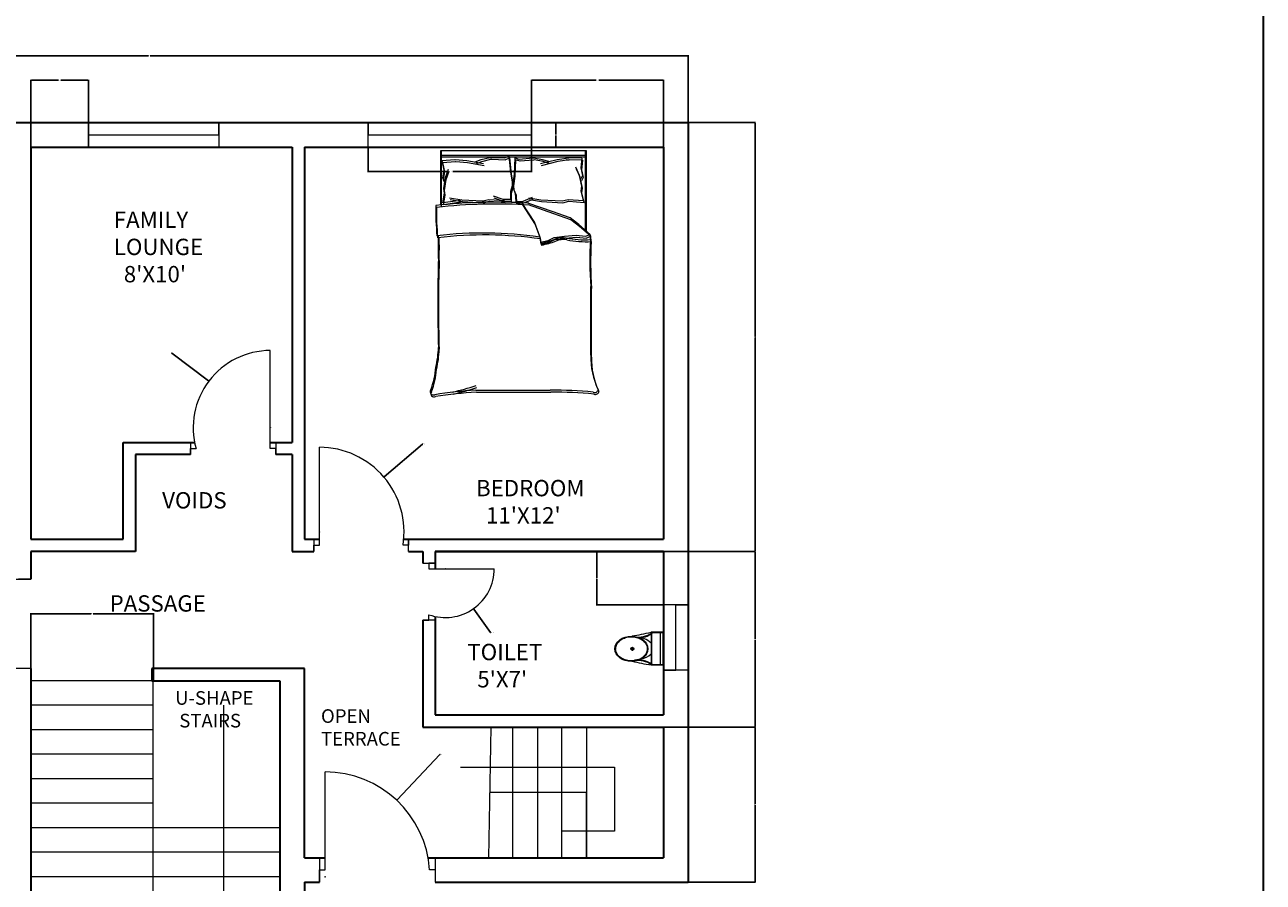
# Model space of a CAD drawing. Units: inches. Extents: x 2067 to 3463, y 1605 to 2723.
# Tile 10 of 10: x 3008 to 3463, y 1879 to 2194. Entities that reach past the tile are written whole.
import ezdxf

# ---------------------------------------------------------------- set-up
doc = ezdxf.new("R2010")
doc.units = ezdxf.units.IN
for name, color, linetype, lineweight in [('A-ANNO-DIMS', 2, 'Continuous', 18), ('A-ANNO-TTLB', 7, 'Continuous', 35), ('A-AREA-IDEN', 7, 'Continuous', 18), ('A-DOOR', 3, 'Continuous', 18), ('A-FLOR-FIXT', 8, 'Continuous', 18), ('A-FLOR-STRS', 7, 'Continuous', 18), ('A-FURN', 8, 'Continuous', 13), ('A-GLAZ', 4, 'Continuous', 18), ('A-WALL', 7, 'Continuous', 35)]:
    doc.layers.add(name, color=color, linetype=linetype, lineweight=lineweight)
doc.styles.get("Standard").update_dxf_attribs({"font": 'arial.ttf'})
doc.dimstyles.get("Standard").update_dxf_attribs({"dimtxt": 0.18, "dimasz": 0.18, "dimexe": 0.18, "dimexo": 0.0625, "dimgap": 0.09, "dimtad": 0, "dimtih": 1, "dimtoh": 1, "dimdec": 4, "dimzin": 0, "dimdsep": 46, "dimtxsty": 'Standard', "dimcen": 0.09, "dimadec": 0, "dimazin": 0, "dimtfac": 1, "dimtdec": 4, "dimtofl": 0, "dimtmove": 0, "dimatfit": 3, "dimfxl": 1, "dimtolj": 1, "dimtzin": 0, "dimarcsym": 0})

# ---------------------------------------------------------------- blocks, each defined once
blk = doc.blocks.new('A$C31115884')
for p, q in [((283, 498), (223, 498)), ((258, 466), (258, 523)), ((0, 200), (0, 0)), ((520, 200), (0, 200)), ((520, 0), (520, 200)), ((510, 54), (0, 54)), ((10, 190), (10, 10)), ((510, 190), (10, 190)), ((10, 10), (510, 10)), ((510, 10), (510, 190)), ((0, 0), (520, 0))]:
    blk.add_line(p, q)
blk.add_circle((256, 496), 23.6)
for centre, radius, start, end in [((2778, -205), 2807, 165.4549, 171.7133), ((-295, 403), 365, 324.2091, 9.3499), ((-295, 403), 375, 324.2091, 9.3499), ((139, 406), 293, 315.8436, 2.6563), ((806, 403), 375, 179.2036, 215.7909), ((806, 403), 365, 170.6501, 215.7909), ((3237, 905), 2807, 188.2867, 194.5451), ((384, 406), 293, 190.2774, 224.1564)]:
    blk.add_arc(centre, radius, start, end)
blk.add_ellipse((256, 510), major_axis=(0, -261), ratio=0.772727)
blk.add_open_spline([(256, 259), (263, 259), (270, 260), (288, 262), (299, 265), (320, 273), (330, 278), (350, 291), (360, 299), (378, 316), (386, 326), (402, 347), (409, 358), (421, 383), (427, 395), (436, 422), (440, 436), (445, 465), (447, 480), (448, 509), (448, 524), (445, 553), (443, 568), (436, 596), (432, 610), (422, 636), (416, 649), (402, 672), (395, 683), (379, 703), (370, 712), (351, 728), (341, 735), (321, 746), (310, 751), (289, 757), (278, 759), (256, 761), (245, 761), (223, 757), (212, 754), (191, 746), (181, 741), (161, 728), (151, 720), (133, 703), (125, 693), (110, 672), (103, 660), (90, 636), (85, 623), (76, 596), (72, 582), (67, 553), (66, 538), (64, 509), (65, 494), (68, 465), (70, 450), (77, 422), (81, 408), (91, 382), (97, 370), (111, 346), (118, 335), (135, 316), (144, 307), (162, 291), (172, 284), (193, 273), (203, 269), (225, 262), (236, 260), (250, 259), (253, 259), (256, 259)], degree=3, knots=[0, 0, 0, 0, 0.110105, 0.110105, 0.285049, 0.285049, 0.459994, 0.459994, 0.634938, 0.634938, 0.809882, 0.809882, 0.984827, 0.984827, 1.159771, 1.159771, 1.334715, 1.334715, 1.50966, 1.50966, 1.684604, 1.684604, 1.859549, 1.859549, 2.034493, 2.034493, 2.209437, 2.209437, 2.384382, 2.384382, 2.559326, 2.559326, 2.73427, 2.73427, 2.909215, 2.909215, 3.084159, 3.084159, 3.259103, 3.259103, 3.434048, 3.434048, 3.608992, 3.608992, 3.783936, 3.783936, 3.958881, 3.958881, 4.133825, 4.133825, 4.30877, 4.30877, 4.483714, 4.483714, 4.658658, 4.658658, 4.833603, 4.833603, 5.008547, 5.008547, 5.183491, 5.183491, 5.358436, 5.358436, 5.53338, 5.53338, 5.708324, 5.708324, 5.883269, 5.883269, 6.058213, 6.058213, 6.233158, 6.233158, 6.283185, 6.283185, 6.283185, 6.283185])
blk = doc.blocks.new('BED-DOUBLE')
for p, q in [((3.86, 70.43), (3.86, 90.57)), ((3.86, 90.57), (57.01, 90.57)), ((3.86, 88.86), (57.01, 88.86)), ((4.12, 89.85), (4.12, 90.57)), ((4.12, 69.72), (4.12, 89.85)), ((4.12, 88.15), (57.26, 88.15)), ((4.33, 86.88), (4.97, 83.34)), ((4.34, 86.85), (9.1, 87.22)), ((4.59, 86.14), (9.35, 86.51)), ((9.1, 87.22), (9.21, 87.2)), ((9.21, 87.2), (13.46, 86.88)), ((9.35, 86.51), (9.47, 86.49)), ((9.47, 86.49), (13.72, 86.17)), ((13.46, 86.88), (19.57, 85.75)), ((16.52, 86.4), (18.77, 87.2)), ((16.77, 85.68), (19.02, 86.49)), ((18.77, 87.2), (21.98, 88)), ((19.02, 86.49), (22.24, 87.29)), ((21.98, 88), (22.34, 88)), ((22.24, 87.29), (22.6, 87.29)), ((22.34, 88), (27.29, 87.84)), ((22.6, 87.29), (27.54, 87.13)), ((27.29, 87.84), (28.89, 88.49)), ((27.54, 87.13), (29.15, 87.77)), ((28.89, 88.49), (29.54, 82.54)), ((29.15, 87.77), (29.79, 81.83)), ((31.11, 87.79), (30.84, 81.82)), ((31.36, 87.08), (31.09, 81.11)), ((32.76, 87.25), (31.11, 87.79)), ((33.01, 86.54), (31.36, 87.08)), ((37.68, 87.72), (32.76, 87.25)), ((37.93, 87.01), (33.01, 86.54)), ((38.04, 87.74), (37.68, 87.72)), ((38.29, 87.03), (37.93, 87.01)), ((41.29, 87.14), (38.04, 87.74)), ((41.55, 86.43), (38.29, 87.03)), ((46.61, 87.15), (40.58, 85.65)), ((43.59, 86.48), (41.29, 87.14)), ((50.83, 87.74), (46.61, 87.15)), ((51.09, 87.03), (46.86, 86.44)), ((55.73, 87.72), (49.72, 87.83)), ((49.72, 87.83), (50.83, 87.74)), ((55.98, 87.01), (49.97, 87.12)), ((49.97, 87.12), (51.09, 87.03)), ((55.73, 87.72), (55.3, 84.15)), ((55.98, 87.01), (55.56, 83.44)), ((57.01, 90.57), (57.01, 60.97)), ((57.01, 90.57), (57.26, 90.57)), ((57.26, 90.57), (57.26, 89.74)), ((57.26, 89.85), (57.26, 60.26)), ((4.97, 83.34), (4.49, 80.45)), ((4.59, 86.17), (5.23, 82.63)), ((5.23, 82.63), (4.75, 79.74)), ((5.62, 80.61), (6.74, 83.66)), ((5.87, 79.9), (7, 82.95)), ((13.72, 86.17), (19.83, 85.04)), ((29.54, 82.54), (30.18, 79)), ((46.86, 86.44), (40.84, 84.94)), ((43.85, 85.77), (41.55, 86.43)), ((54.83, 81.38), (53.52, 84.36)), ((55.09, 80.67), (53.77, 83.65)), ((55.3, 84.15), (55.97, 81.29)), ((55.56, 83.44), (56.22, 80.58)), ((4.49, 80.45), (5.13, 79.32)), ((4.75, 79.74), (5.39, 78.61)), ((4.97, 76.59), (5.62, 80.61)), ((5.23, 75.88), (5.87, 79.9)), ((30.18, 77.55), (29.54, 75.46)), ((29.79, 81.83), (30.43, 78.29)), ((30.18, 79), (30.18, 77.55)), ((30.84, 81.82), (30.42, 78.25)), ((30.42, 78.25), (30.51, 76.8)), ((30.43, 78.29), (30.43, 76.84)), ((31.09, 81.11), (30.67, 77.54)), ((30.67, 77.54), (30.76, 76.09)), ((55.73, 77.41), (54.83, 81.38)), ((55.98, 76.7), (55.09, 80.67)), ((55.97, 81.29), (55.39, 80.13)), ((55.51, 75.63), (55.73, 77.41)), ((56.22, 80.58), (55.65, 79.42)), ((4.65, 71.28), (5.3, 74.82)), ((4.91, 70.57), (5.55, 74.11)), ((5.3, 74.82), (4.97, 76.59)), ((5.55, 74.11), (5.23, 75.88)), ((7.1, 73.19), (11.58, 72.44)), ((26.8, 72.48), (23.31, 73.69)), ((27.06, 71.77), (23.56, 72.98)), ((29.54, 75.46), (29.54, 72.48)), ((30.43, 76.84), (29.79, 74.75)), ((29.79, 74.75), (29.79, 71.77)), ((30.51, 76.8), (31.28, 74.76)), ((30.76, 76.09), (31.54, 74.05)), ((31.28, 74.76), (31.47, 71.78)), ((31.54, 74.05), (31.72, 71.07)), ((34.19, 71.95), (37.61, 73.38)), ((36.21, 73.19), (40.7, 72.44)), ((56.38, 72.14), (55.51, 75.63)), ((55.77, 74.92), (55.98, 76.7)), ((56.63, 71.43), (55.77, 74.92)), ((10.32, 72.09), (4.65, 71.28)), ((10.57, 71.37), (4.91, 70.57)), ((7.35, 72.48), (11.83, 71.73)), ((11.58, 72.44), (10.32, 72.09)), ((11.83, 71.73), (10.57, 71.37)), ((11.58, 72.44), (19.38, 71.97)), ((11.83, 71.73), (19.63, 71.25)), ((19.38, 71.97), (21.56, 72.58)), ((19.63, 71.25), (21.81, 71.87)), ((21.56, 72.58), (27.26, 72.14)), ((21.81, 71.87), (27.52, 71.43)), ((29.54, 72.48), (26.8, 72.48)), ((29.79, 71.77), (27.06, 71.77)), ((31.47, 71.78), (34.19, 71.95)), ((31.72, 71.07), (34.45, 71.24)), ((33.65, 71.23), (38.31, 64.01)), ((33.9, 70.52), (38.56, 63.3)), ((34.45, 71.24), (37.86, 72.67)), ((45.2, 67.97), (35.92, 71.23)), ((45.45, 67.26), (36.18, 70.52)), ((36.47, 72.48), (40.95, 71.73)), ((40.7, 72.44), (48.49, 71.97)), ((40.95, 71.73), (48.74, 71.25)), ((48.49, 71.97), (50.67, 72.58)), ((48.74, 71.25), (50.92, 71.87)), ((50.67, 72.58), (56.38, 72.14)), ((50.92, 71.87), (56.63, 71.43)), ((38.31, 64.01), (40.2, 59.02)), ((51.4, 65.74), (45.2, 67.97)), ((51.65, 65.02), (45.45, 67.26)), ((54.67, 63.33), (51.4, 65.74)), ((54.92, 62.61), (51.65, 65.02)), ((38.56, 63.3), (40.46, 58.31)), ((49.33, 59.02), (53.64, 59.37)), ((53.64, 59.37), (57.08, 59.02)), ((58.79, 59.71), (54.67, 63.33)), ((59.04, 59), (54.92, 62.61)), ((57.08, 59.02), (58.79, 59.71)), ((58.88, 57.77), (58.79, 59.71, 4.3)), ((40.2, 59.02), (40.55, 56.79)), ((40.46, 58.31), (40.8, 56.07)), ((40.55, 56.79), (43.3, 57.47)), ((40.8, 56.07), (43.56, 56.76)), ((43.3, 57.47), (45.54, 58.51)), ((43.56, 56.76), (45.8, 57.8)), ((45.54, 58.51), (49.33, 59.02)), ((45.8, 57.8), (49.58, 58.31)), ((49.58, 58.31), (53.89, 58.66)), ((53.89, 58.66), (57.33, 58.31)), ((57.33, 58.31), (59.04, 59)), ((59.13, 57.06), (59.04, 59, 4.3)), ((16.75, 2.44), (44.12, 2.44)), ((17, 1.73), (44.38, 1.73))]:
    blk.add_line(p, q)
for centre, radius, start, end in [((94.7, 68.22), 92.64, 178.7218, 185.604), ((23.75, -111.88), 183.45, 86.0865, 96.7821), ((94.95, 67.51), 92.64, 178.7218, 185.604), ((24.01, -112.59), 183.45, 86.0865, 96.7821), ((19.74, -83.26), 143.47, 81.7845, 96.9006), ((20, -83.97), 143.47, 81.7845, 96.9006), ((-186.05, 55.9), 189.16, 358.4762, 1.0082), ((-185.79, 55.19), 189.16, 358.4762, 1.0082), ((40.74, 56.72), 0.205, 160.2464, 271.1377), ((34.64, 88.92), 32.98, 280.6617, 289.8806), ((40.99, 56.01), 0.205, 160.2464, 271.1377), ((34.9, 88.21), 32.98, 280.6617, 289.8806), ((48.64, 51.57), 6.92, 78.6608, 113.7384), ((48.9, 50.86), 6.92, 78.6608, 113.7384), ((57.08, 97.97), 40.24, 259.8763, 272.5657), ((57.33, 97.26), 40.24, 259.8763, 272.5657), ((202.68, 50.18), 144, 176.9791, 183.8365), ((202.94, 49.47), 144, 176.9791, 183.8365), ((539.13, 34.28), 536.33, 178.2277, 181.7185), ((539.38, 33.57), 536.33, 178.2277, 181.7185), ((-5013.77, 15.15), 5072.83, 0.00217, 0.28689), ((-5013.52, 14.44), 5072.83, 0.00217, 0.28689), ((-29.91, 18.82), 32.95, 346.0648, 358.9113), ((-29.66, 18.11), 32.95, 346.0648, 358.9113), ((84.69, 14.21), 25.65, 177.4714, 206.4681), ((84.94, 13.5), 25.65, 177.4714, 206.4681), ((-24.09, 12.42), 26.2, 337.9751, 356.652), ((-23.83, 11.71), 26.2, 337.9751, 356.652), ((1.21, 1.92), 1.21, 146.1736, 293.4781), ((1.46, 1.21), 1.21, 146.1736, 293.4781), ((23.83, -132.77), 135.4, 92.9958, 99.4091), ((24.08, -133.48), 135.4, 92.9958, 99.4091), ((-19.15, 116.93), 118.38, 283.3832, 287.7053), ((-18.9, 116.22), 118.38, 283.3832, 287.7053), ((45.76, -145.49), 147.94, 84.4998, 90.6351), ((46.02, -146.2), 147.94, 84.4998, 90.6351), ((60.5, 2.86), 1.23, 242.6588, 356.02), ((60.76, 2.15), 1.23, 242.6588, 356.02)]:
    blk.add_arc(centre, radius, start, end)
blk = doc.blocks.new('WIN-PLAN-24-OFFSET')
for p, q in [((0, 24), (9, 24)), ((9, 24), (4.5, 24)), ((4.5, 24), (4.5, 0)), ((4.5, 0), (0, 0)), ((0, 0), (9, 0))]:
    blk.add_line(p, q)
blk = doc.blocks.new('WIN-PLAN-48-OFFSET')
for p, q in [((0, 9), (0, 0)), ((48, 4.5), (48, 9)), ((48, 9), (48, 0)), ((0, 0), (0, 4.5)), ((0, 4.5), (48, 4.5))]:
    blk.add_line(p, q)
blk = doc.blocks.new('WIN-PLAN-60-ALIGNED')
for p, q in [((0, 0), (0, 9)), ((0, 9), (0, 4.5)), ((60, 4.5), (60, 9)), ((60, 9), (60, 0)), ((0, 4.5), (60, 4.5))]:
    blk.add_line(p, q)
blk = doc.blocks.new('*D24')
at = {"layer": 'A-ANNO-DIMS', "color": 0, "lineweight": -2, "transparency": 16777216}
for p, q in [((3134.41, 2149.17), (3134.41, 2140.05)), ((3194.41, 2149.17), (3194.41, 2140.05)), ((3134.59, 2140.23), (3163.3, 2140.23)), ((3194.23, 2140.23), (3165.53, 2140.23))]:
    blk.add_line(p, q, dxfattribs=at)
at = {"layer": 'A-ANNO-DIMS', "color": 0, "transparency": 16777216}
for points in [[(3134.59, 2140.26), (3134.59, 2140.2), (3134.41, 2140.23)], [(3194.23, 2140.26), (3194.23, 2140.2), (3194.41, 2140.23)]]:
    blk.add_solid(points, dxfattribs=at)
at = {"layer": 'Defpoints', "color": 0, "transparency": 16777216}
for p in [(3134.41, 2149.23), (3194.41, 2149.23), (3194.41, 2140.23)]:
    blk.add_point(p, dxfattribs=at)
at = {"layer": 'A-ANNO-DIMS', "color": 0, "transparency": 16777216, "insert": (3164.41, 2140.23), "char_height": 0.18, "attachment_point": 5}
blk.add_mtext('\\A1;WINDOW 60 TYP.', dxfattribs=at)
blk = doc.blocks.new('*D25')
at = {"layer": 'A-ANNO-DIMS', "color": 0, "lineweight": -2, "transparency": 16777216}
for p, q in [((3194.48, 2158.23), (3203.59, 2158.23)), ((3203.41, 2158.05), (3203.41, 2153.91)), ((3203.41, 2149.41), (3203.41, 2153.55)), ((3194.48, 2149.23), (3203.59, 2149.23))]:
    blk.add_line(p, q, dxfattribs=at)
at = {"layer": 'A-ANNO-DIMS', "color": 0, "transparency": 16777216}
for points in [[(3203.38, 2158.05), (3203.44, 2158.05), (3203.41, 2158.23)], [(3203.38, 2149.41), (3203.44, 2149.41), (3203.41, 2149.23)]]:
    blk.add_solid(points, dxfattribs=at)
at = {"layer": 'Defpoints', "color": 0, "transparency": 16777216}
for p in [(3194.41, 2158.23), (3203.41, 2158.23), (3194.41, 2149.23)]:
    blk.add_point(p, dxfattribs=at)
at = {"layer": 'A-ANNO-DIMS', "color": 0, "transparency": 16777216, "insert": (3203.41, 2153.73), "char_height": 0.18, "attachment_point": 5}
blk.add_mtext('\\A1;9 TYP.', dxfattribs=at)
blk = doc.blocks.new('*D50')
at = {"layer": 'A-ANNO-DIMS', "color": 0, "lineweight": -2, "transparency": 16777216}
for p, q in [((2856, 2158.29), (2856, 2183.01)), ((2856.18, 2182.83), (3053.71, 2182.83)), ((3251.82, 2182.83), (3054.29, 2182.83)), ((3252, 2158.29), (3252, 2183.01))]:
    blk.add_line(p, q, dxfattribs=at)
at = {"layer": 'A-ANNO-DIMS', "color": 0, "transparency": 16777216}
for points in [[(2856.18, 2182.86), (2856.18, 2182.8), (2856, 2182.83)], [(3251.82, 2182.86), (3251.82, 2182.8), (3252, 2182.83)]]:
    blk.add_solid(points, dxfattribs=at)
at = {"layer": 'Defpoints', "color": 0, "transparency": 16777216}
for p in [(3252, 2182.83), (2856, 2158.23), (3252, 2158.23)]:
    blk.add_point(p, dxfattribs=at)
at = {"layer": 'A-ANNO-DIMS', "color": 0, "transparency": 16777216, "insert": (3054, 2182.83), "char_height": 0.18, "attachment_point": 5}
blk.add_mtext('\\A1;396', dxfattribs=at)
blk = doc.blocks.new('*D58')
at = {"layer": 'A-ANNO-DIMS', "color": 0, "lineweight": -2, "transparency": 16777216}
for p, q in [((3252.06, 2158.23), (3276.78, 2158.23)), ((3276.6, 2158.05), (3276.6, 2079.66)), ((3276.6, 2000.91), (3276.6, 2079.3)), ((3243.06, 2000.73), (3276.78, 2000.73))]:
    blk.add_line(p, q, dxfattribs=at)
at = {"layer": 'A-ANNO-DIMS', "color": 0, "transparency": 16777216}
for points in [[(3276.57, 2158.05), (3276.63, 2158.05), (3276.6, 2158.23)], [(3276.57, 2000.91), (3276.63, 2000.91), (3276.6, 2000.73)]]:
    blk.add_solid(points, dxfattribs=at)
at = {"layer": 'Defpoints', "color": 0, "transparency": 16777216}
for p in [(3252, 2158.23), (3243, 2000.73), (3276.6, 2000.73)]:
    blk.add_point(p, dxfattribs=at)
at = {"layer": 'A-ANNO-DIMS', "color": 0, "transparency": 16777216, "insert": (3276.6, 2079.48), "char_height": 0.18, "attachment_point": 5}
blk.add_mtext('\\A1;157.5', dxfattribs=at)
blk = doc.blocks.new('*D59')
at = {"layer": 'A-ANNO-DIMS', "color": 0, "lineweight": -2, "transparency": 16777216}
for p, q in [((3243.06, 2000.73), (3276.78, 2000.73)), ((3276.6, 2000.55), (3276.6, 1968.66)), ((3276.6, 1936.41), (3276.6, 1968.3)), ((3243.06, 1936.23), (3276.78, 1936.23))]:
    blk.add_line(p, q, dxfattribs=at)
at = {"layer": 'A-ANNO-DIMS', "color": 0, "transparency": 16777216}
for points in [[(3276.57, 2000.55), (3276.63, 2000.55), (3276.6, 2000.73)], [(3276.57, 1936.41), (3276.63, 1936.41), (3276.6, 1936.23)]]:
    blk.add_solid(points, dxfattribs=at)
at = {"layer": 'Defpoints', "color": 0, "transparency": 16777216}
for p in [(3243, 2000.73), (3243, 1936.23), (3276.6, 1936.23)]:
    blk.add_point(p, dxfattribs=at)
at = {"layer": 'A-ANNO-DIMS', "color": 0, "transparency": 16777216, "insert": (3276.6, 1968.48), "char_height": 0.18, "attachment_point": 5}
blk.add_mtext('\\A1;64.5', dxfattribs=at)
blk = doc.blocks.new('*D60')
at = {"layer": 'A-ANNO-DIMS', "color": 0, "lineweight": -2, "transparency": 16777216}
for p, q in [((3243.06, 1936.23), (3276.78, 1936.23)), ((3276.6, 1936.05), (3276.6, 1907.91)), ((3276.6, 1879.41), (3276.6, 1907.55)), ((3252.06, 1879.23), (3276.78, 1879.23))]:
    blk.add_line(p, q, dxfattribs=at)
at = {"layer": 'A-ANNO-DIMS', "color": 0, "transparency": 16777216}
for points in [[(3276.57, 1936.05), (3276.63, 1936.05), (3276.6, 1936.23)], [(3276.57, 1879.41), (3276.63, 1879.41), (3276.6, 1879.23)]]:
    blk.add_solid(points, dxfattribs=at)
at = {"layer": 'Defpoints', "color": 0, "transparency": 16777216}
for p in [(3243, 1936.23), (3276.6, 1936.23), (3252, 1879.23)]:
    blk.add_point(p, dxfattribs=at)
at = {"layer": 'A-ANNO-DIMS', "color": 0, "transparency": 16777216, "insert": (3276.6, 1907.73), "char_height": 0.18, "attachment_point": 5}
blk.add_mtext('\\A1;57', dxfattribs=at)
blk = doc.blocks.new('*D63')
at = {"layer": 'A-ANNO-DIMS', "color": 0, "lineweight": -2, "transparency": 16777216}
for p, q in [((3010.5, 2149.29), (3010.5, 2174.01)), ((3010.68, 2173.83), (3020.59, 2173.83)), ((3031.44, 2173.83), (3021.52, 2173.83)), ((3031.62, 2149.29), (3031.62, 2174.01))]:
    blk.add_line(p, q, dxfattribs=at)
at = {"layer": 'A-ANNO-DIMS', "color": 0, "transparency": 16777216}
for points in [[(3010.68, 2173.86), (3010.68, 2173.8), (3010.5, 2173.83)], [(3031.44, 2173.86), (3031.44, 2173.8), (3031.62, 2173.83)]]:
    blk.add_solid(points, dxfattribs=at)
at = {"layer": 'Defpoints', "color": 0, "transparency": 16777216}
for p in [(3031.62, 2173.83), (3010.5, 2149.23), (3031.62, 2149.23)]:
    blk.add_point(p, dxfattribs=at)
at = {"layer": 'A-ANNO-DIMS', "color": 0, "transparency": 16777216, "insert": (3021.06, 2173.83), "char_height": 0.18, "attachment_point": 5}
blk.add_mtext('\\A1;21.117', dxfattribs=at)
blk = doc.blocks.new('*D64')
at = {"layer": 'A-ANNO-DIMS', "color": 0, "lineweight": -2, "transparency": 16777216}
for p, q in [((3194.41, 2149.29), (3194.41, 2174.01)), ((3194.59, 2173.83), (3218.24, 2173.83)), ((3242.82, 2173.83), (3219.17, 2173.83)), ((3243, 2149.29), (3243, 2174.01))]:
    blk.add_line(p, q, dxfattribs=at)
at = {"layer": 'A-ANNO-DIMS', "color": 0, "transparency": 16777216}
for points in [[(3194.59, 2173.86), (3194.59, 2173.8), (3194.41, 2173.83)], [(3242.82, 2173.86), (3242.82, 2173.8), (3243, 2173.83)]]:
    blk.add_solid(points, dxfattribs=at)
at = {"layer": 'Defpoints', "color": 0, "transparency": 16777216}
for p in [(3243, 2173.83), (3194.41, 2149.23), (3243, 2149.23)]:
    blk.add_point(p, dxfattribs=at)
at = {"layer": 'A-ANNO-DIMS', "color": 0, "transparency": 16777216, "insert": (3218.71, 2173.83), "char_height": 0.18, "attachment_point": 5}
blk.add_mtext('\\A1;48.585', dxfattribs=at)
blk = doc.blocks.new('*D65')
at = {"layer": 'A-ANNO-DIMS', "color": 0, "lineweight": -2, "transparency": 16777216}
for p, q in [((3242.94, 2000.73), (3218.22, 2000.73)), ((3218.4, 2000.55), (3218.4, 1991.09)), ((3218.4, 1981.26), (3218.4, 1990.73)), ((3242.94, 1981.08), (3218.22, 1981.08))]:
    blk.add_line(p, q, dxfattribs=at)
at = {"layer": 'A-ANNO-DIMS', "color": 0, "transparency": 16777216}
for points in [[(3218.37, 2000.55), (3218.43, 2000.55), (3218.4, 2000.73)], [(3218.37, 1981.26), (3218.43, 1981.26), (3218.4, 1981.08)]]:
    blk.add_solid(points, dxfattribs=at)
at = {"layer": 'Defpoints', "color": 0, "transparency": 16777216}
for p in [(3218.4, 2000.73), (3243, 2000.73), (3243, 1981.08)]:
    blk.add_point(p, dxfattribs=at)
at = {"layer": 'A-ANNO-DIMS', "color": 0, "transparency": 16777216, "insert": (3218.4, 1990.91), "char_height": 0.18, "attachment_point": 5}
blk.add_mtext('\\A1;19.647', dxfattribs=at)
blk = doc.blocks.new('*D66')
at = {"layer": 'A-ANNO-DIMS', "color": 0, "lineweight": -2, "transparency": 16777216}
for p, q in [((3010.5, 1953.32), (3010.5, 1978.03)), ((3010.68, 1977.85), (3032.6, 1977.85)), ((3055.31, 1977.85), (3033.39, 1977.85)), ((3055.49, 1953.32), (3055.49, 1978.03))]:
    blk.add_line(p, q, dxfattribs=at)
at = {"layer": 'A-ANNO-DIMS', "color": 0, "transparency": 16777216}
for points in [[(3010.68, 1977.88), (3010.68, 1977.82), (3010.5, 1977.85)], [(3055.31, 1977.88), (3055.31, 1977.82), (3055.49, 1977.85)]]:
    blk.add_solid(points, dxfattribs=at)
at = {"layer": 'Defpoints', "color": 0, "transparency": 16777216}
for p in [(3055.49, 1977.85), (3010.5, 1953.25), (3055.49, 1953.25)]:
    blk.add_point(p, dxfattribs=at)
at = {"layer": 'A-ANNO-DIMS', "color": 0, "transparency": 16777216, "insert": (3032.99, 1977.85), "char_height": 0.18, "attachment_point": 5}
blk.add_mtext('\\A1;44.99', dxfattribs=at)
blk = doc.blocks.new('*D107')
at = {"layer": 'A-ANNO-DIMS', "color": 0, "lineweight": -2, "transparency": 16777216}
for p, q in [((3160.7, 1926.18), (3145.03, 1909.46)), ((3160.88, 1926.18), (3160.7, 1926.18)), ((3118.49, 1881.23), (3118.67, 1881.23)), ((3118.58, 1881.14), (3118.58, 1881.32))]:
    blk.add_line(p, q, dxfattribs=at)
at = {"layer": 'A-ANNO-DIMS', "color": 0, "transparency": 16777216}
blk.add_solid([(3145, 1909.48), (3145.05, 1909.44), (3144.9, 1909.32)], dxfattribs=at)
at = {"layer": 'Defpoints', "color": 0, "transparency": 16777216}
for p in [(3144.9, 1909.32), (3118.58, 1881.23)]:
    blk.add_point(p, dxfattribs=at)
at = {"layer": 'A-ANNO-DIMS', "color": 0, "transparency": 16777216, "insert": (3161.29, 1926.18), "char_height": 0.18, "attachment_point": 5}
blk.add_mtext('\\A1;R38.5', dxfattribs=at)
blk = doc.blocks.new('*D109')
at = {"layer": 'A-ANNO-DIMS', "color": 0, "lineweight": -2, "transparency": 16777216}
for p, q in [((3154.38, 2040.18), (3140.32, 2028.18)), ((3154.56, 2040.18), (3154.38, 2040.18)), ((3116.43, 2007.88), (3116.61, 2007.88)), ((3116.52, 2007.79), (3116.52, 2007.97))]:
    blk.add_line(p, q, dxfattribs=at)
at = {"layer": 'A-ANNO-DIMS', "color": 0, "transparency": 16777216}
blk.add_solid([(3140.3, 2028.21), (3140.34, 2028.16), (3140.18, 2028.07)], dxfattribs=at)
at = {"layer": 'Defpoints', "color": 0, "transparency": 16777216}
for p in [(3140.18, 2028.07), (3116.52, 2007.88)]:
    blk.add_point(p, dxfattribs=at)
at = {"layer": 'A-ANNO-DIMS', "color": 0, "transparency": 16777216, "insert": (3154.95, 2040.18), "char_height": 0.18, "attachment_point": 5}
blk.add_mtext('\\A1;R31.1', dxfattribs=at)
blk = doc.blocks.new('*D111')
at = {"layer": 'A-ANNO-DIMS', "color": 0, "lineweight": -2, "transparency": 16777216}
for p, q in [((3062.15, 2073.6), (3062.33, 2073.6)), ((3062.33, 2073.6), (3075.74, 2063.42)), ((3098.39, 2046.17), (3098.57, 2046.17)), ((3098.48, 2046.08), (3098.48, 2046.26))]:
    blk.add_line(p, q, dxfattribs=at)
at = {"layer": 'A-ANNO-DIMS', "color": 0, "transparency": 16777216}
blk.add_solid([(3075.76, 2063.45), (3075.72, 2063.4), (3075.88, 2063.31)], dxfattribs=at)
at = {"layer": 'Defpoints', "color": 0, "transparency": 16777216}
for p in [(3075.88, 2063.31), (3098.48, 2046.17)]:
    blk.add_point(p, dxfattribs=at)
at = {"layer": 'A-ANNO-DIMS', "color": 0, "transparency": 16777216, "insert": (3061.67, 2073.6), "char_height": 0.18, "attachment_point": 5}
blk.add_mtext('\\A1;R28.36', dxfattribs=at)
blk = doc.blocks.new('*D114')
at = {"layer": 'A-ANNO-DIMS', "color": 0, "lineweight": -2, "transparency": 16777216}
for p, q in [((3162.7, 1994.4), (3162.88, 1994.4)), ((3162.79, 1994.31), (3162.79, 1994.49)), ((3179.34, 1970.91), (3173.24, 1979.57)), ((3179.52, 1970.91), (3179.34, 1970.91))]:
    blk.add_line(p, q, dxfattribs=at)
at = {"layer": 'A-ANNO-DIMS', "color": 0, "transparency": 16777216}
blk.add_solid([(3173.26, 1979.59), (3173.21, 1979.55), (3173.13, 1979.72)], dxfattribs=at)
at = {"layer": 'Defpoints', "color": 0, "transparency": 16777216}
for p in [(3162.79, 1994.4), (3173.13, 1979.72)]:
    blk.add_point(p, dxfattribs=at)
at = {"layer": 'A-ANNO-DIMS', "color": 0, "transparency": 16777216, "insert": (3180.07, 1970.91), "char_height": 0.18, "attachment_point": 5}
blk.add_mtext('\\A1;R17.955', dxfattribs=at)

msp = doc.modelspace()

# ---------------------------------------------------------------- linework, layer by layer
at = {"layer": 'A-ANNO-TTLB'}
msp.add_lwpolyline([(2067.2624, 2722.6321), (3463.3053, 2722.6321), (3463.3053, 1605.3918), (2067.2624, 1605.3918)], close=True, dxfattribs=at)
at = {"layer": 'A-DOOR'}
for p, q in [((3098.478, 2062.5341), (3098.478, 2074.5341)), ((3098.478, 2038.5341), (3098.478, 2062.5341)), ((3069.166, 2040.7841), (3069.166, 2036.2841)), ((3100.478, 2040.7841), (3100.478, 2036.2841)), ((3116.5225, 2002.9809), (3116.5225, 2038.9809)), ((3069.166, 2036.2841), (3069.166, 2038.5341)), ((3069.166, 2038.5341), (3071.166, 2038.5341)), ((3100.478, 2038.5341), (3098.478, 2038.5341)), ((3100.478, 2036.2841), (3100.478, 2038.5341)), ((3114.5225, 2005.2309), (3114.5225, 2000.7309)), ((3114.5225, 2000.7309), (3114.5225, 2002.9809)), ((3114.5225, 2002.9809), (3116.5225, 2002.9809)), ((3149.2364, 2002.9809), (3147.2364, 2002.9809)), ((3149.2364, 2000.7309), (3149.2364, 2005.2309)), ((3149.2364, 2005.2309), (3149.2364, 2002.9809)), ((3154.4994, 1996.398), (3158.9994, 1996.398)), ((3158.9994, 1996.398), (3156.7494, 1996.398)), ((3156.7494, 1996.398), (3156.7494, 1994.398)), ((3156.7494, 1994.398), (3180.7494, 1994.398)), ((3001.4994, 1990.4993), (3010.4994, 1990.4993)), ((3010.4994, 1990.4993), (3005.9994, 1990.4993)), ((3158.9994, 1975.4909), (3154.4994, 1975.4909)), ((3154.4994, 1975.4909), (3156.7494, 1975.4909)), ((3156.7494, 1975.4909), (3156.7494, 1977.4909)), ((3010.4994, 1957.7531), (3001.4994, 1957.7531)), ((3118.5782, 1883.7309), (3118.5782, 1919.7309)), ((3116.5782, 1888.2309), (3116.5782, 1879.2309)), ((3158.9994, 1888.2309), (3158.9994, 1879.2309)), ((3116.5782, 1879.2309), (3116.5782, 1883.7309)), ((3116.5782, 1883.7309), (3118.5782, 1883.7309)), ((3158.9994, 1883.7309), (3156.9994, 1883.7309))]:
    msp.add_line(p, q, dxfattribs=at)
for centre, radius, start, end in [((3098.478, 2046.1737), 28.3604, 90, 195.62716), ((3116.5225, 2007.8788), 31.102, 350.939279, 90), ((3162.7942, 1994.398), 17.9552, 250.326439, 360), ((3118.5782, 1881.2283), 38.5026, 3.726746, 90)]:
    msp.add_arc(centre, radius, start, end, dxfattribs=at)
at = {"layer": 'A-FLOR-STRS'}
for p, q in [((3055.4865, 1953.2531), (3010.4994, 1953.2531)), ((3055.4865, 1809.2531), (3055.4865, 1953.2531)), ((3055.4865, 1944.2531), (3010.4994, 1944.2531)), ((3081.2715, 1944.2531), (3081.2715, 1786.8304)), ((3055.4865, 1935.2531), (3010.4994, 1935.2531)), ((3179.4811, 1936.2309), (3178.625, 1888.2309)), ((3187.625, 1888.2309), (3187.625, 1936.2309)), ((3187.625, 1936.2309), (3196.625, 1936.2309)), ((3196.625, 1936.2309), (3196.625, 1888.2309)), ((3205.625, 1888.2309), (3205.625, 1936.2309)), ((3205.625, 1936.2309), (3214.625, 1936.2309)), ((3214.625, 1936.2309), (3214.625, 1888.2309)), ((3055.4865, 1926.2531), (3010.4994, 1926.2531)), ((3168.393, 1921.4335), (3224.9811, 1921.4335)), ((3224.9811, 1921.4335), (3224.9811, 1897.969)), ((3055.4865, 1917.2531), (3010.4994, 1917.2531)), ((3214.625, 1912.2309), (3179.053, 1912.2309)), ((3214.625, 1888.2309), (3214.625, 1912.2309)), ((3055.4865, 1908.2531), (3010.4994, 1908.2531)), ((3101.9994, 1899.2531), (3010.4994, 1899.2531)), ((3224.9811, 1897.969), (3205.625, 1897.969)), ((3101.9994, 1890.2531), (3010.4994, 1890.2531)), ((3178.625, 1888.2309), (3187.625, 1888.2309)), ((3196.625, 1888.2309), (3205.625, 1888.2309)), ((3101.9994, 1881.2531), (3010.4994, 1881.2531))]:
    msp.add_line(p, q, dxfattribs=at)
at = {"layer": 'A-GLAZ'}
msp.add_line((3251.9994, 1957.0835), (3251.9994, 1957.0835), dxfattribs=at)
at = {"layer": 'A-WALL'}
for p, q in [((2855.9994, 2158.2309), (3251.9994, 2158.2309)), ((3251.9994, 2158.2309), (3251.9994, 1879.2309)), ((3010.4994, 2149.2309), (3010.4994, 2005.2309)), ((3010.4994, 2149.2309), (3106.4994, 2149.2309)), ((3106.4994, 2149.2309), (3106.4994, 2040.7841)), ((3110.9994, 2149.2309), (3110.9994, 2005.2309)), ((3110.9994, 2149.2309), (3242.9994, 2149.2309)), ((3242.9994, 2149.2309), (3242.9994, 2005.2309)), ((3044.4521, 2040.7841), (3070.6345, 2040.7841)), ((3044.4521, 2005.2309), (3044.4521, 2040.7841)), ((3044.4521, 2040.7841), (3048.9521, 2040.7841)), ((3098.478, 2040.7841), (3106.4994, 2040.7841)), ((3069.166, 2036.2841), (3048.9521, 2036.2841)), ((3048.9521, 2036.2841), (3048.9521, 2000.7309)), ((3106.4994, 2036.2841), (3100.478, 2036.2841)), ((3106.4994, 2036.2841), (3106.4994, 2000.7309)), ((3010.4994, 2005.2309), (3044.4521, 2005.2309)), ((3110.9994, 2005.2309), (3116.5225, 2005.2309)), ((3147.5116, 2005.2309), (3242.9994, 2005.2309)), ((3048.9521, 2000.7309), (3010.4994, 2000.7309)), ((3010.4994, 2000.7309), (3010.4994, 1996.2309)), ((3010.4994, 2000.7309), (3010.4994, 1990.4993)), ((3106.4994, 2000.7309), (3114.5225, 2000.7309)), ((3149.2364, 2000.7309), (3154.4994, 2000.7309)), ((3154.4994, 2000.7309), (3154.4994, 1996.398)), ((3242.9994, 2000.7309), (3158.9994, 2000.7309)), ((3158.9994, 2000.7309), (3158.9994, 1994.398)), ((3158.9994, 2000.7309), (3242.9994, 2000.7309)), ((3242.9994, 2000.7309), (3242.9994, 2000.7309)), ((3242.9994, 2000.7309), (3242.9994, 1940.7309)), ((3154.4994, 1975.4909), (3154.4994, 1936.2309)), ((3158.9994, 1976.8484), (3158.9994, 1940.7309)), ((3010.4994, 1957.7531), (3010.4994, 1771.2309)), ((3101.9994, 1957.7531), (3054.9518, 1957.7531)), ((3054.9518, 1957.7531), (3054.9518, 1953.2531)), ((3110.9994, 1957.7531), (3101.9994, 1957.7531)), ((3110.9994, 1888.2309), (3110.9994, 1957.7531)), ((3054.9518, 1953.2531), (3101.9994, 1953.2531)), ((3101.9994, 1953.2531), (3101.9994, 1888.2309)), ((3158.9994, 1940.7309), (3242.9994, 1940.7309)), ((3154.4994, 1936.2309), (3158.9994, 1936.2309)), ((3158.9994, 1936.2309), (3242.9994, 1936.2309)), ((3242.9994, 1936.2309), (3242.9994, 1888.2309)), ((3101.9994, 1888.2309), (3101.9994, 1771.2309)), ((3110.9994, 1888.2309), (3118.5782, 1888.2309)), ((3156.4387, 1888.2309), (3242.9994, 1888.2309)), ((3110.9994, 1879.2309), (3116.5782, 1879.2309)), ((3110.9994, 1879.2309), (3110.9994, 1771.2309)), ((3158.9994, 1879.2309), (3242.9994, 1879.2309)), ((3242.9994, 1879.2309), (3251.9994, 1879.2309))]:
    msp.add_line(p, q, dxfattribs=at)

# ---------------------------------------------------------------- block references
at = {"layer": 'A-FLOR-FIXT', "xscale": 0.0231892354596934, "yscale": 0.0231892354596934, "zscale": 0.0231892354596934, "rotation": 89.99999999999996}
msp.add_blockref('A$C31115884', (3242.9994, 1959.0276), dxfattribs=at)
at = {"layer": 'A-FURN'}
msp.add_blockref('BED-DOUBLE', (3157.2077, 2057.4856), dxfattribs=at)
at = {"layer": 'A-GLAZ'}
for name, p in [('WIN-PLAN-48-OFFSET', (3031.6162, 2149.231)), ('WIN-PLAN-60-ALIGNED', (3134.414, 2149.231))]:
    msp.add_blockref(name, p, dxfattribs=at)
at = {"layer": 'A-GLAZ', "rotation": 180}
msp.add_blockref('WIN-PLAN-24-OFFSET', (3251.9991, 1981.0834), dxfattribs=at)

# ---------------------------------------------------------------- texts
at = {"layer": 'A-AREA-IDEN', "attachment_point": 1}
for s, width, insert, char_height in [("FAMILY\\PLOUNGE\\P  8'X10'", 137.479312, (3040.9712, 2125.5932), 6), ("BEDROOM\\P  11'X12'", 98.598369, (3174.0704, 2026.9921), 6), ('VOIDS', 44.06277, (3058.7263, 2022.5132), 6), ('PASSAGE', 45.174144, (3039.4165, 1984.6363), 6), ("TOILET\\P  5'X7'", 39.932546, (3170.8634, 1966.7896), 6), ('U-SHAPE\\P STAIRS', 35.601018, (3063.5002, 1949.4105), 5), ('OPEN \\PTERRACE', 91.66607, (3117.0958, 1942.7629), 5)]:
    msp.add_mtext_dynamic_manual_height_columns(s, width=width, gutter_width=12.5, heights=[0], dxfattribs=dict(at, insert=insert, char_height=char_height))

# ---------------------------------------------------------------- dimensions: what is measured, and where the dimension line sits
at = {"layer": 'A-ANNO-DIMS'}
for base, p1, p2, override, picture, middle in [((3251.9994, 2182.8309), (2855.9994, 2158.2309), (3251.9994, 2158.2309), {"dimdec": 0, "dimlfac": 1, "dimrnd": 0, "dimzin": 0, "dimdsep": 46, "dimlunit": 2}, '*D50', (3053.9994, 2182.8309)), ((3031.6164, 2173.8309), (3010.4994, 2149.2309), (3031.6164, 2149.2309), {"dimdec": 3, "dimlfac": 1, "dimrnd": 0, "dimzin": 0, "dimdsep": 46, "dimlunit": 2}, '*D63', (3021.0579, 2173.8309)), ((3242.9994, 2173.8309), (3194.4143, 2149.2309), (3242.9994, 2149.2309), {"dimdec": 3, "dimlfac": 1, "dimrnd": 0, "dimzin": 0, "dimdsep": 46, "dimlunit": 2}, '*D64', (3218.7069, 2173.8309)), ((3055.4865, 1977.8531), (3010.4994, 1953.2531), (3055.4865, 1953.2531), {"dimdec": 2, "dimlfac": 1, "dimrnd": 0, "dimzin": 0, "dimdsep": 46, "dimlunit": 2}, '*D66', (3032.993, 1977.8531))]:
    dim = msp.add_linear_dim(base=base, p1=p1, p2=p2, dimstyle='Standard', override=override, dxfattribs=at)
    dim.commit()
    dim.dimension.update_dxf_attribs({"geometry": picture, "text_midpoint": middle})
dim = msp.add_linear_dim(base=(3203.4143, 2158.2309), p1=(3194.4143, 2149.2309), p2=(3194.4143, 2158.2309), angle=90, text='<> TYP.', dimstyle='Standard', override={"dimdec": 0, "dimlfac": 1, "dimrnd": 0, "dimzin": 0, "dimdsep": 46, "dimlunit": 2}, dxfattribs=at)
dim.commit()
dim.dimension.update_dxf_attribs({"geometry": '*D25', "text_midpoint": (3203.4143, 2153.7309)})
for base, p1, p2, override, picture, middle in [((3276.5994, 2000.7309), (3251.9994, 2158.2309), (3242.9994, 2000.7309), {"dimdec": 1, "dimlfac": 1, "dimrnd": 0, "dimzin": 0, "dimdsep": 46, "dimlunit": 2}, '*D58', (3276.5994, 2079.4809)), ((3218.3994, 2000.7309), (3242.9994, 1981.0835), (3242.9994, 2000.7309), {"dimdec": 3, "dimlfac": 1, "dimrnd": 0, "dimzin": 0, "dimdsep": 46, "dimlunit": 2}, '*D65', (3218.3994, 1990.9072)), ((3276.5994, 1936.2309), (3242.9994, 2000.7309), (3242.9994, 1936.2309), {"dimdec": 1, "dimlfac": 1, "dimrnd": 0, "dimzin": 0, "dimdsep": 46, "dimlunit": 2}, '*D59', (3276.5994, 1968.4809)), ((3276.5994, 1936.2309), (3251.9994, 1879.2309), (3242.9994, 1936.2309), {"dimdec": 0, "dimlfac": 1, "dimrnd": 0, "dimzin": 0, "dimdsep": 46, "dimlunit": 2}, '*D60', (3276.5994, 1907.7309))]:
    dim = msp.add_linear_dim(base=base, p1=p1, p2=p2, angle=90, dimstyle='Standard', override=override, dxfattribs=at)
    dim.commit()
    dim.dimension.update_dxf_attribs({"geometry": picture, "text_midpoint": middle})
dim = msp.add_linear_dim(base=(3194.4143, 2140.2309), p1=(3134.4143, 2149.2309), p2=(3194.4143, 2149.2309), text='WINDOW <> TYP.', dimstyle='Standard', override={"dimdec": 0, "dimlfac": 1, "dimrnd": 0, "dimzin": 0, "dimdsep": 46, "dimlunit": 2}, dxfattribs=at)
dim.commit()
dim.dimension.update_dxf_attribs({"geometry": '*D24', "text_midpoint": (3164.4143, 2140.2309)})
for center, mpoint, override, picture, middle in [((3098.478, 2046.1737), (3075.884, 2063.315), {"dimdec": 2, "dimlfac": 1, "dimrnd": 0, "dimzin": 0, "dimdsep": 46, "dimlunit": 2}, '*D111', (3061.6679, 2073.5997)), ((3116.5225, 2007.8788), (3140.1834, 2028.0654), {"dimdec": 1, "dimlfac": 1, "dimrnd": 0, "dimzin": 0, "dimdsep": 46, "dimlunit": 2}, '*D109', (3154.9525, 2040.1773)), ((3162.7942, 1994.398), (3173.1347, 1979.7194), {"dimdec": 3, "dimlfac": 1, "dimrnd": 0, "dimzin": 0, "dimdsep": 46, "dimlunit": 2}, '*D114', (3180.0695, 1970.9122)), ((3118.5782, 1881.2283), (3144.9038, 1909.3248), {"dimdec": 1, "dimlfac": 1, "dimrnd": 0, "dimzin": 0, "dimdsep": 46, "dimlunit": 2}, '*D107', (3161.2897, 1926.1827))]:
    dim = msp.add_radius_dim(center=center, mpoint=mpoint, dimstyle='Standard', override=override, dxfattribs=at)
    dim.commit()
    dim.dimension.update_dxf_attribs({"geometry": picture, "text_midpoint": middle, "dimtype": 164})

doc.saveas('drawing.dxf')
